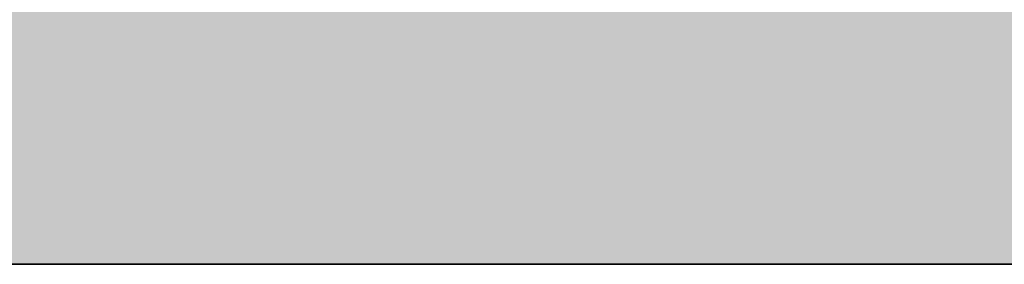
# Model space of a CAD drawing. Units: inches. Extents: x 2083 to 3317, y 1141 to 2115.
# Tile 157 of 256: x 3126.955939 to 3126.958245, y 1263.26136 to 1263.261932. Entities that reach past the tile are written whole.
import ezdxf

# ---------------------------------------------------------------- set-up
doc = ezdxf.new("R2010")
doc.units = ezdxf.units.IN
doc.layers.add('A-ANNO-DIMS', color=2, linetype='Continuous', lineweight=18)
doc.layers.add('A-WALL', color=7, linetype='Continuous', lineweight=35)
doc.layers.add('A-WALL-PATT', color=251, linetype='Continuous', lineweight=13, true_color=0x636466)
doc.styles.get("Standard").update_dxf_attribs({"font": 'arial.ttf'})
doc.dimstyles.new('ISO-25', dxfattribs={"dimtxt": 12, "dimasz": 12, "dimexe": 1.25, "dimexo": 0.625, "dimtad": 1, "dimlunit": 3, "dimtxsty": 'Standard', "dimcen": 2.5, "dimadec": 0, "dimazin": 0, "dimtfac": 1, "dimtmove": 0, "dimatfit": 3, "dimfxl": 1, "dimarcsym": 0})

# ---------------------------------------------------------------- blocks, each defined once
blk = doc.blocks.new('*D10')
at = {"layer": 'A-ANNO-DIMS', "color": 0, "lineweight": -2, "transparency": 16777216}
for p, q in [((2862.9597832, 1262.6363601), (2862.9597832, 1201.3844498)), ((3126.9597832, 1262.6363601), (3126.9597832, 1201.3844498)), ((2874.9597832, 1202.6344498), (3114.9597832, 1202.6344498))]:
    blk.add_line(p, q, dxfattribs=at)
at = {"layer": 'A-ANNO-DIMS', "color": 0, "transparency": 16777216}
for points in [[(2874.9597832, 1204.6344498), (2874.9597832, 1200.6344498), (2862.9597832, 1202.6344498)], [(3114.9597832, 1204.6344498), (3114.9597832, 1200.6344498), (3126.9597832, 1202.6344498)]]:
    blk.add_solid(points, dxfattribs=at)
at = {"layer": 'Defpoints', "color": 0, "transparency": 16777216}
for p in [(2862.9597832, 1263.2613601), (3126.9597832, 1263.2613601), (3126.9597832, 1202.6344498)]:
    blk.add_point(p, dxfattribs=at)
at = {"layer": 'A-ANNO-DIMS', "color": 0, "transparency": 16777216, "insert": (2994.9597832, 1209.2840064), "char_height": 12, "attachment_point": 5}
blk.add_mtext("22'", dxfattribs=at)

msp = doc.modelspace()

# ---------------------------------------------------------------- hatches: boundary and pattern name
at = {"layer": 'A-WALL-PATT'}
h = msp.add_hatch(color=256, dxfattribs=at)
h.dxf.hatch_style = 1
h.paths.add_polyline_path([(3126.9597832, 2020.7613601), (2748.9597832, 2020.7613601), (2604.9597832, 2020.7613601), (2226.9597832, 2020.7613601), (2226.9597832, 1702.7613601), (2466.9597832, 1702.7613601), (2466.9597832, 1582.7613601), (2418.9597832, 1582.7613601), (2418.9597832, 1477.7613601), (2226.9597832, 1477.7613601), (2226.9597832, 1263.2613601), (2544.9597832, 1263.2613601), (2544.9597832, 1411.7613601), (2604.9597832, 1411.7613601), (2685.9597832, 1411.7613601), (2685.9597832, 1420.7613601), (2604.9597832, 1420.7613601), (2604.9597832, 1573.7613601), (2604.9597832, 1702.7613601), (2604.9597832, 2011.7613601), (2748.9597832, 2011.7613601), (2748.9597832, 1702.7613601), (2862.9597832, 1702.7613601), (2862.9597832, 1621.7613601), (2871.9597832, 1621.7613601), (2871.9597832, 1702.7613601), (2883.9597832, 1702.7613601), (2883.9597832, 1706.9394595, -0.026459), (2883.9597832, 1711.7613601), (2757.9597832, 1711.7613601), (2757.9597832, 1807.7613601), (2787.9597832, 1807.7613601), (2787.9597832, 1812.2613601), (2757.9597832, 1812.2613601), (2757.9597832, 2011.7613601), (2877.9597832, 2011.7613601), (2877.9597832, 1812.2613601), (2847.9597832, 1812.2613601), (2847.9597832, 1807.7613601), (2889.8357425, 1807.7613601), (2889.8357425, 1812.2613601), (2882.4597832, 1812.2613601), (2882.4597832, 2011.7613601), (3117.9597832, 2011.7613601), (3117.9597832, 1812.2613601), (2937.8357425, 1812.2613601), (2937.8357425, 1807.7613601), (2995.7097832, 1807.7613601), (2995.7097832, 1796.1176655), (3000.2097832, 1796.1176655), (3000.2097832, 1807.7613601), (3117.9597832, 1807.7613601), (3117.9597832, 1711.7613601), (3000.2097832, 1711.7613601), (3000.2097832, 1760.1176655), (2998.5727047, 1760.1176655, -0.020711), (2995.7097832, 1760.1176655), (2995.7097832, 1711.7613601), (2931.9597832, 1711.7613601), (2931.9597832, 1702.7613601), (3126.9597832, 1702.7613601)])
h.paths.add_polyline_path([(2471.4597832, 2011.7613601), (2471.4597832, 1810.0113601), (2462.7169357, 1810.0113601), (2462.7169357, 1805.5113601), (2505.9597832, 1805.5113601), (2505.9597832, 1810.0113601), (2475.9597832, 1810.0113601), (2475.9597832, 2011.7613601), (2595.9597832, 2011.7613601), (2595.9597832, 1810.0113601), (2565.9597832, 1810.0113601), (2565.9597832, 1805.5113601), (2595.9597832, 1805.5113601), (2595.9597832, 1711.7613601), (2235.9597832, 1711.7613601), (2235.9597832, 1805.5113601), (2353.7097832, 1805.5113601), (2353.7097832, 1796.0541624), (2358.2097832, 1796.0541624), (2358.2097832, 1805.5113601), (2414.7169357, 1805.5113601), (2414.7169357, 1810.0113601), (2235.9597832, 1810.0113601), (2235.9597832, 2011.7613601)], flags=16)
h.paths.add_polyline_path([(2270.2047343, 1994.6100082), (2270.2047343, 1970.6100082), (2246.2047343, 1970.6100082), (2246.2047343, 1994.6100082)], flags=0)
edge = h.paths.add_edge_path(flags=0)
edge.add_ellipse((2332.027391, 1899.7981761), major_axis=(-3.0429938, 3.0429938), ratio=0.16825245, start_angle=-161.3321656, end_angle=-156.3071136, ccw=False)
edge.add_ellipse((2333.0820373, 1898.7435297), major_axis=(-1.0546463, 1.0546463), ratio=0.453532097, start_angle=-123.371019, end_angle=-94.1591066)
edge = h.paths.add_edge_path(flags=0)
edge.add_ellipse((2332.027391, 1968.8762897), major_axis=(3.0429938, 3.0429938), ratio=0.16825245, start_angle=18.6678344, end_angle=23.6928864)
edge.add_spline(control_points=[(2332.9255964, 1970.6911045), (2332.2267681, 1970.3360997), (2330.8937087, 1969.6589054), (2328.4130803, 1970.9321376), (2327.2039345, 1967.7487119), (2324.7095965, 1969.9555886), (2322.5328223, 1967.012354), (2320.0128462, 1971.2958124), (2317.6803077, 1968.1578449), (2316.0405263, 1967.1020468), (2315.4269045, 1966.8096022)], knot_values=[0, 0, 0, 0, 2.267059, 4.324559, 6.685584, 8.878641, 11.121502, 14.300359, 17.755284, 19.732645, 19.732645, 19.732645, 19.732645], degree=3, periodic=0)
edge.add_ellipse((2332.027391, 1968.8762897), major_axis=(3.0429938, 3.0429938), ratio=0.16825245, start_angle=18.6678344, end_angle=23.6928864, ccw=False)
edge.add_ellipse((2333.0820373, 1969.930936), major_axis=(1.0546463, 1.0546463), ratio=0.453532097, start_angle=56.628981, end_angle=85.8408934, ccw=False)
edge = h.paths.add_edge_path(flags=0)
edge.add_spline(control_points=[(2296.4282874, 1967.9879081), (2293.6278045, 1965.3363137), (2287.7036238, 1959.727094), (2299.7438601, 1949.9956993), (2294.5325909, 1935.6685275), (2290.5732281, 1920.6035119), (2293.3941244, 1909.9736911), (2296.1854073, 1904.9665431)], knot_values=[0.099185, 0.099185, 0.099185, 0.099185, 0.345301, 0.619822, 0.982653, 1.386093, 1.810555, 1.810555, 1.810555, 1.810555], degree=3, periodic=0)
edge.add_spline(control_points=[(2296.1854073, 1904.9665431), (2297.3835817, 1902.6193002), (2298.0009694, 1901.9493116), (2298.5529698, 1901.4681549)], knot_values=[0.006246, 0.006246, 0.006246, 0.006246, 0.055476, 0.055476, 0.055476, 0.055476], degree=3, periodic=0)
edge.add_spline(control_points=[(2298.5529698, 1901.4681549), (2297.2586121, 1900.9232238), (2295.2252939, 1900.2321257), (2293.0602287, 1900.6142053), (2292.1014227, 1900.788415), (2292.0895776, 1900.790568)], knot_values=[0.312835, 0.312835, 0.312835, 0.312835, 0.40178, 0.474987, 0.475903, 0.475903, 0.475903, 0.475903], degree=3, periodic=0)
edge.add_arc((2292.7936464, 1904.6641088), 3.9370079, 215.4208969, 259.6981795, ccw=False)
edge.add_spline(control_points=[(2289.5853139, 1902.3823039), (2289.4766524, 1902.5350874), (2289.3684805, 1902.6880353), (2289.2608648, 1902.8411699)], knot_values=[0.102872, 0.102872, 0.102872, 0.102872, 0.116896, 0.116896, 0.116896, 0.116896], degree=3, periodic=0)
edge.add_spline(control_points=[(2289.2608648, 1902.8411699), (2288.6866042, 1902.5501922), (2287.6400477, 1902.0199025), (2285.8813368, 1901.8739536), (2283.8529717, 1901.5043521), (2281.7199871, 1899.7105375), (2278.4669913, 1899.492942), (2276.1571361, 1901.8832022), (2272.2589526, 1899.8040711), (2267.7776054, 1901.8431828), (2262.2438819, 1900.1840326), (2257.414927, 1901.7820606), (2254.318374, 1900.7261196), (2253.1782849, 1900.3373431)], knot_values=[0, 0, 0, 0, 1.907977, 3.477176, 5.261074, 7.972851, 11.680248, 13.717921, 16.939592, 22.789562, 27.502503, 33.595215, 37.145618, 37.145618, 37.145618, 37.145618], degree=3, periodic=0)
edge.add_line((2253.1782849, 1900.3373431), (2250.2442397, 1902.8411699))
edge.add_line((2250.2442397, 1902.8411699), (2250.2442397, 1965.8332959))
edge.add_line((2250.2442397, 1965.8332959), (2253.1782849, 1968.3371226))
edge.add_spline(control_points=[(2253.1782849, 1968.3371226), (2254.318374, 1967.9483462), (2257.414927, 1966.8924051), (2262.2438819, 1968.4904332), (2267.7776054, 1966.8312829), (2271.5267301, 1968.5372172), (2273.8759143, 1967.8282895), (2274.2067012, 1967.7276424)], knot_values=[0, 0, 0, 0, 0.09018, 0.244935, 0.364644, 0.513233, 0.537855, 0.537855, 0.537855, 0.537855], degree=3, periodic=0)
edge.add_arc((2274.3528869, 1963.7933495), 3.9370079, 72.0511336, 92.1279492, ccw=False)
edge.add_arc((2281.2969331, 1985.2300027), 18.5962982, 252.05113361, 288.56572166)
edge.add_arc((2292.3167172, 1956.0288805), 12.6460805, 71.02678788, 113.77821843, ccw=False)
edge = h.paths.add_edge_path(flags=0)
edge.add_spline(control_points=[(2274.8994147, 1951.8561946), (2275.066156, 1951.6165924), (2275.2326866, 1951.3765878), (2275.3979871, 1951.1358545)], knot_values=[1.409916, 1.409916, 1.409916, 1.409916, 1.43159, 1.43159, 1.43159, 1.43159], degree=3, periodic=0)
edge.add_spline(control_points=[(2275.3979871, 1951.1358545), (2275.7921055, 1950.5618854), (2276.1792311, 1949.9837745), (2276.5455462, 1949.3971029)], knot_values=[1.358238, 1.358238, 1.358238, 1.358238, 1.409916, 1.409916, 1.409916, 1.409916], degree=3, periodic=0)
edge.add_line((2276.5455462, 1949.3971029), (2277.437289, 1947.8621847))
edge.add_spline(control_points=[(2277.437289, 1947.8621847), (2276.3038341, 1945.6731147), (2274.6396979, 1942.4268817), (2274.631615, 1938.0938998), (2272.7991237, 1930.8515498), (2274.3564261, 1943.8970461), (2275.9476814, 1947.9233558), (2276.5455462, 1949.3971029)], knot_values=[0.005632, 0.005632, 0.005632, 0.005632, 0.186014, 0.266002, 0.357087, 0.59639, 0.739732, 0.739732, 0.739732, 0.739732], degree=3, periodic=0)
edge.add_spline(control_points=[(2276.5455462, 1949.3971029), (2276.1792311, 1949.9837745), (2275.7921055, 1950.5618854), (2275.3979871, 1951.1358545)], knot_values=[1.358238, 1.358238, 1.358238, 1.358238, 1.409916, 1.409916, 1.409916, 1.409916], degree=3, periodic=0)
edge.add_spline(control_points=[(2275.3979871, 1951.1358545), (2274.9425002, 1950.0804523), (2274.2077604, 1948.0252718), (2273.9346018, 1944.8514774), (2272.4685341, 1937.6274891), (2273.4662155, 1945.6964663), (2274.7006154, 1951.0594725), (2274.8994147, 1951.8561946)], knot_values=[0.104364, 0.104364, 0.104364, 0.104364, 0.189636, 0.269624, 0.36071, 0.600013, 0.644622, 0.644622, 0.644622, 0.644622], degree=3, periodic=0)
h.paths.add_polyline_path([(2269.1675139, 1963.1275729, -0.357527), (2268.170633, 1960.9763695, -0.092561), (2268.170633, 1939.4363249, -0.357527), (2269.1675139, 1937.2851215, -0.357527), (2267.0163105, 1938.2820024, -0.164785), (2254.6855813, 1938.2820024, -0.357527), (2252.5343779, 1937.2851215, -0.357527), (2253.5312587, 1939.4363249, -0.092561), (2253.5312587, 1960.9763695, -0.357527), (2252.5343779, 1963.1275729, -0.357527), (2254.6855813, 1962.130692, -0.164785), (2267.0163105, 1962.130692, -0.357527)], flags=0)
h.paths.add_polyline_path([(2248.8740679, 1967.8017998), (2248.8740679, 1957.0277095), (2249.4577833, 1957.0277095), (2249.4577833, 1911.6467562), (2248.8740679, 1911.6467562), (2248.8740679, 1900.8726659), (2246.5118632, 1900.8726659, 0.197327), (2244.1496584, 1902.4568734), (2244.1496584, 1966.2175923, 0.197327), (2246.5118632, 1967.8017998)], flags=0)
h.paths.add_polyline_path([(2269.1675139, 1931.3893442, -0.357527), (2268.170633, 1929.2381408, -0.092561), (2268.170633, 1907.6980962, -0.357527), (2269.1675139, 1905.5468928, -0.357527), (2267.0163105, 1906.5437737, -0.164785), (2254.6855813, 1906.5437737, -0.357527), (2252.5343779, 1905.5468928, -0.357527), (2253.5312587, 1907.6980962, -0.092561), (2253.5312587, 1929.2381408, -0.357527), (2252.5343779, 1931.3893442, -0.357527), (2254.6855813, 1930.3924634, -0.164785), (2267.0163105, 1930.3924634, -0.357527)], flags=0)
edge = h.paths.add_edge_path(flags=0)
edge.add_spline(control_points=[(2276.1968578, 1906.7237016), (2276.1681442, 1909.0289278), (2276.1140492, 1913.371852), (2270.5984171, 1924.9249783), (2273.9051746, 1919.0127787), (2275.9217115, 1916.2620626), (2275.4745699, 1912.4021495), (2277.2578735, 1910.3806206), (2276.6960436, 1908.2250358), (2276.6462176, 1906.8130226), (2276.6178249, 1906.0084068)], knot_values=[0, 0, 0, 0, 8.61026, 16.221274, 18.843057, 23.804898, 27.440828, 29.356102, 31.203478, 33.650687, 33.650687, 33.650687, 33.650687], degree=3, periodic=0)
edge.add_spline(control_points=[(2276.6178249, 1906.0084068), (2276.6233131, 1905.6241436), (2276.4977381, 1904.6286608), (2275.4417789, 1903.8547251), (2274.9373144, 1903.0804497), (2274.8590804, 1902.8411699)], knot_values=[0.156488, 0.156488, 0.156488, 0.156488, 0.184398, 0.231376, 0.250598, 0.250598, 0.250598, 0.250598], degree=3, periodic=0)
edge.add_line((2274.8590804, 1902.8411699), (2276.50598, 1902.8411699))
edge.add_spline(control_points=[(2276.50598, 1902.8411699), (2276.7883084, 1903.0849395), (2277.6650711, 1904.1251958), (2278.2495378, 1904.340738), (2277.6538719, 1908.5273866), (2278.15567, 1906.2278078), (2278.100464, 1905.2859484), (2278.8466748, 1904.0690054), (2277.8567853, 1903.4149482), (2277.8741909, 1902.9910497), (2277.9035616, 1902.8411699)], knot_values=[0.059574, 0.059574, 0.059574, 0.059574, 0.080753, 0.103741, 0.16972, 0.176036, 0.207137, 0.240474, 0.262341, 0.27366, 0.27366, 0.27366, 0.27366], degree=3, periodic=0)
edge.add_line((2277.9035616, 1902.8411699), (2280.0298255, 1902.8411699))
edge.add_spline(control_points=[(2280.0298255, 1902.8411699), (2279.8882214, 1903.088398), (2279.4992571, 1903.9815512), (2280.1522839, 1905.9393491), (2278.103615, 1909.6577572), (2279.7623946, 1907.185285), (2280.3279002, 1904.8748608), (2280.4851086, 1903.4895904), (2281.4632687, 1903.2494323), (2281.7583431, 1902.9364967), (2281.8340361, 1902.8411699)], knot_values=[0.013856, 0.013856, 0.013856, 0.013856, 0.034874, 0.088867, 0.107879, 0.126738, 0.158714, 0.193757, 0.217487, 0.226722, 0.226722, 0.226722, 0.226722], degree=3, periodic=0)
edge.add_spline(control_points=[(2281.8340361, 1902.8411699), (2281.7875348, 1902.8267029), (2281.6470224, 1902.7829881), (2281.3955272, 1902.85949), (2281.088077, 1902.9852418), (2280.7206826, 1903.060902), (2280.3334513, 1903.0257257), (2280.1247668, 1902.898879), (2280.0298255, 1902.8411699)], knot_values=[0, 0, 0, 0, 0.14413, 0.435517, 0.749276, 1.153046, 1.548371, 1.878348, 1.878348, 1.878348, 1.878348], degree=3, periodic=0)
edge.add_line((2280.0298255, 1902.8411699), (2277.9035616, 1902.8411699))
edge.add_spline(control_points=[(2277.9035616, 1902.8411699), (2277.892855, 1902.7958553), (2277.865396, 1902.6796374), (2277.6074793, 1902.6874828), (2277.2740503, 1902.8006999), (2276.8379209, 1902.6197745), (2276.5838074, 1902.7892611), (2276.50598, 1902.8411699)], knot_values=[0, 0, 0, 0, 0.127189, 0.326199, 0.628009, 1.24357, 1.515331, 1.515331, 1.515331, 1.515331], degree=3, periodic=0)
edge.add_line((2276.50598, 1902.8411699), (2274.8590804, 1902.8411699))
edge.add_spline(control_points=[(2274.8590804, 1902.8411699), (2274.8144367, 1902.8985868), (2274.7251297, 1903.013446), (2274.4934765, 1903.1189684), (2274.2442854, 1902.9605386), (2273.9371207, 1903.1849416), (2273.6140395, 1902.9831428), (2273.4083164, 1902.8830449), (2273.322254, 1902.8411699)], knot_values=[0, 0, 0, 0, 0.21843, 0.436957, 0.687977, 0.990379, 1.398396, 1.69185, 1.69185, 1.69185, 1.69185], degree=3, periodic=0)
edge.add_spline(control_points=[(2273.322254, 1902.8411699), (2273.6167403, 1903.445692), (2274.2739977, 1904.5382529), (2276.0272387, 1904.5737017), (2276.2069634, 1906.5836372), (2276.1968578, 1906.7237016)], knot_values=[0.012227, 0.012227, 0.012227, 0.012227, 0.059472, 0.106218, 0.134458, 0.134458, 0.134458, 0.134458], degree=3, periodic=0)
h.paths.add_polyline_path([(2270.7760538, 1897.7898284), (2270.7760538, 1873.7898284), (2246.7760538, 1873.7898284), (2246.7760538, 1897.7898284)], flags=0)
h.paths.add_polyline_path([(2353.7097832, 1760.0050593), (2353.7097832, 1760.0541624), (2358.2097832, 1760.0541624, -0.033729)], flags=0)
h.paths.add_polyline_path([(2321.8191188, 1737.5291862), (2341.9953271, 1737.5291862, -0.414214), (2343.2032727, 1736.3212406), (2343.2032727, 1721.0205964, -0.414214), (2341.9953271, 1719.8126508), (2321.8191188, 1719.8126508, -0.414214), (2320.6111732, 1721.0205964), (2320.6111732, 1736.3212406, -0.414214)], flags=0)
h.paths.add_polyline_path([(2324.2350099, 1736.3212406), (2339.5794359, 1736.3212406, -0.414214), (2341.9953271, 1733.9053494), (2341.9953271, 1725.4497302, -0.414214), (2339.5794359, 1723.033839), (2333.6805885, 1723.033839), (2333.8453172, 1722.0454666, -0.870646), (2335.4253988, 1721.8258934, -0.767327), (2333.922694, 1721.4232449), (2331.2910241, 1721.4232449, -0.767327), (2329.7883193, 1721.8258934, -0.870646), (2331.3684009, 1722.0454666), (2331.5331296, 1723.033839), (2324.2350099, 1723.033839, -0.414214), (2321.8191188, 1725.4497302), (2321.8191188, 1733.9053494, -0.414214)], flags=0)
h.paths.add_polyline_path([(2570.4837892, 1928.6154443), (2589.6837892, 1928.6154443), (2590.1688286, 1928.6154443), (2590.1688286, 1904.9933971), (2570.4837892, 1904.9933971)], flags=0)
h.paths.add_polyline_path([(2574.4473242, 1927.2638215, -1), (2572.8288357, 1927.2638215, -1)], flags=0)
h.paths.add_polyline_path([(2573.0898665, 1926.9408768), (2573.925032, 1927.7760423), (2574.1477428, 1927.5533315), (2573.3125773, 1926.718166)], flags=0)
h.paths.add_polyline_path([(2578.7790648, 1919.7296175, -1), (2571.5916632, 1919.7296175, -1)], flags=0)
h.paths.add_polyline_path([(2578.385364, 1919.7296175, -1), (2571.985364, 1919.7296175, -1)], flags=0)
h.paths.add_polyline_path([(2331.5957638, 1729.4762156, -1), (2333.6179542, 1729.4762156, -1)], flags=0)
h.paths.add_polyline_path([(2578.0342282, 1927.2638215, -1), (2576.4157396, 1927.2638215, -1)], flags=0)
h.paths.add_polyline_path([(2576.6888513, 1927.5310886), (2576.9115621, 1927.7537993), (2577.7467276, 1926.9186339), (2577.5240168, 1926.6959231)], flags=0)
h.paths.add_polyline_path([(2578.1390648, 1909.8595388, -1), (2572.2316632, 1909.8595388, -1)], flags=0)
h.paths.add_polyline_path([(2577.745364, 1909.8595388, -1), (2572.625364, 1909.8595388, -1)], flags=0)
h.paths.add_polyline_path([(2583.7977179, 1927.2638215, -1), (2582.1792294, 1927.2638215, -1)], flags=0)
h.paths.add_polyline_path([(2582.7186487, 1927.7537993), (2583.5538142, 1926.9186339), (2583.3311034, 1926.6959231), (2582.4959379, 1927.5310886)], flags=0)
h.paths.add_polyline_path([(2582.4959379, 1927.5310886), (2582.7186487, 1927.7537993), (2583.5538142, 1926.9186339), (2583.3311034, 1926.6959231)], flags=0)
h.paths.add_polyline_path([(2587.7390648, 1920.5296175, -1), (2581.8316632, 1920.5296175, -1)], flags=0)
h.paths.add_polyline_path([(2587.345364, 1920.5296175, -1), (2582.225364, 1920.5296175, -1)], flags=0)
h.paths.add_polyline_path([(2587.3846219, 1927.2638215, -1), (2585.7661333, 1927.2638215, -1)], flags=0)
h.paths.add_polyline_path([(2586.0819925, 1926.9802469), (2586.917158, 1927.8154124), (2587.1398688, 1927.5927016), (2586.3047033, 1926.7575361)], flags=0)
h.paths.add_polyline_path([(2588.3790648, 1910.6595388, -1), (2581.1916632, 1910.6595388, -1)], flags=0)
h.paths.add_polyline_path([(2587.985364, 1910.6595388, -1), (2581.585364, 1910.6595388, -1)], flags=0)
h.paths.add_polyline_path([(2417.1677288, 1729.4778955), (2437.3439372, 1729.4778955, -0.414214), (2438.5518828, 1728.2699499), (2438.5518828, 1712.9693057, -0.414214), (2437.3439372, 1711.7613601), (2417.1677288, 1711.7613601, -0.414214), (2415.9597832, 1712.9693057), (2415.9597832, 1728.2699499, -0.414214)], flags=0)
h.paths.add_polyline_path([(2419.58362, 1728.2699499), (2434.928046, 1728.2699499, -0.414214), (2437.3439372, 1725.8540587), (2437.3439372, 1717.3984395, -0.414214), (2434.928046, 1714.9825483), (2429.0291985, 1714.9825483), (2429.1939273, 1713.9941758, -0.870646), (2430.7740089, 1713.7746027, -0.767327), (2429.2713041, 1713.3719542), (2426.6396342, 1713.3719542, -0.767327), (2425.1369294, 1713.7746027, -0.870646), (2426.717011, 1713.9941758), (2426.8817397, 1714.9825483), (2419.58362, 1714.9825483, -0.414214), (2417.1677288, 1717.3984395), (2417.1677288, 1725.8540587, -0.414214)], flags=0)
h.paths.add_polyline_path([(2419.58362, 1728.2699499), (2434.928046, 1728.2699499, -0.414214), (2437.3439372, 1725.8540587), (2437.3439372, 1717.3984395, -0.414214), (2434.928046, 1714.9825483), (2429.0291985, 1714.9825483), (2428.3581177, 1719.0090337), (2427.5528206, 1719.0090337), (2426.8817397, 1714.9825483), (2419.58362, 1714.9825483, -0.414214), (2417.1677288, 1717.3984395), (2417.1677288, 1725.8540587, -0.414214)], flags=0)
h.paths.add_polyline_path([(2426.9443739, 1721.4249248, -1), (2428.9665643, 1721.4249248, -1)], flags=0)
h.paths.add_polyline_path([(2475.9597832, 1702.7613601), (2595.9597832, 1702.7613601), (2595.9597832, 1582.7613601), (2475.9597832, 1582.7613601)], flags=16)
h.paths.add_polyline_path([(2427.9597832, 1573.7613601), (2595.9597832, 1573.7613601), (2595.9597832, 1468.7613601), (2595.9597832, 1420.7613601), (2384.4597832, 1420.7613601), (2384.4597832, 1468.7613601), (2427.9597832, 1468.7613601)], flags=16)
h.paths.add_polyline_path([(2379.9597832, 1468.7613601), (2379.9597832, 1420.7613601), (2235.9597832, 1420.7613601), (2235.9597832, 1468.7613601)], flags=16)
h.paths.add_polyline_path([(2317.8159962, 1466.695767), (2337.9922045, 1466.695767, -0.414214), (2339.2001501, 1465.4878214), (2339.2001501, 1450.1871771, -0.414214), (2337.9922045, 1448.9792315), (2317.8159962, 1448.9792315, -0.414214), (2316.6080506, 1450.1871771), (2316.6080506, 1465.4878214, -0.414214)], flags=0)
h.paths.add_polyline_path([(2320.2318874, 1465.4878214), (2335.5763133, 1465.4878214, -0.414214), (2337.9922045, 1463.0719302), (2337.9922045, 1454.616311, -0.414214), (2335.5763133, 1452.2004198), (2329.6774659, 1452.2004198), (2329.8421946, 1451.2120473, -0.870646), (2331.4222762, 1450.9924742, -0.767327), (2329.9195714, 1450.5898257), (2327.2879015, 1450.5898257, -0.767327), (2325.7851967, 1450.9924742, -0.870646), (2327.3652783, 1451.2120473), (2327.530007, 1452.2004198), (2320.2318874, 1452.2004198, -0.414214), (2317.8159962, 1454.616311), (2317.8159962, 1463.0719302, -0.414214)], flags=0)
h.paths.add_polyline_path([(2320.2318874, 1465.4878214), (2335.5763133, 1465.4878214, -0.414214), (2337.9922045, 1463.0719302), (2337.9922045, 1454.616311, -0.414214), (2335.5763133, 1452.2004198), (2329.6774659, 1452.2004198), (2329.006385, 1456.2269051), (2328.2010879, 1456.2269051), (2327.530007, 1452.2004198), (2320.2318874, 1452.2004198, -0.414214), (2317.8159962, 1454.616311), (2317.8159962, 1463.0719302, -0.414214)], flags=0)
h.paths.add_polyline_path([(2327.5926413, 1458.6427963, -1), (2329.6148317, 1458.6427963, -1)], flags=0)
h.paths.add_polyline_path([(2244.4117436, 1433.3404531), (2241.9209449, 1433.3404531, -0.414214), (2240.0178562, 1435.2435418), (2240.0178562, 1440.9528078, -0.414211), (2241.920925, 1442.8558965), (2244.4117436, 1442.8558965, -1.976472)], flags=0)
h.paths.add_polyline_path([(2245.3568884, 1434.3975358, -0.414214), (2245.3568884, 1441.7988138, -2.144098)], flags=0)
h.paths.add_polyline_path([(2535.9597832, 1416.2613601), (2535.9597832, 1272.2613601), (2235.9597832, 1272.2613601), (2235.9597832, 1416.2613601)], flags=16)
h.paths.add_polyline_path([(2260.1195614, 1384.2928413), (2260.1195614, 1362.0386487), (2237.8653688, 1362.0386487), (2237.8653688, 1384.2928413)], flags=0)
edge = h.paths.add_edge_path(flags=0)
edge.add_line((2318.2518466, 1362.0932983), (2318.1457968, 1362.0009726))
edge.add_ellipse((2317.4451158, 1360.4310442), major_axis=(2.8216404, 2.8216404), ratio=0.16825245, start_angle=18.6678344, end_angle=20.9481273, ccw=False)
edge.add_ellipse((2318.4230451, 1361.4089735), major_axis=(0.9779293, 0.9779293), ratio=0.453532097, start_angle=56.628981, end_angle=70.2262012, ccw=False)
edge = h.paths.add_edge_path(flags=0)
edge.add_line((2319.1073699, 1295.5710784), (2319.0150442, 1295.6771282))
edge.add_ellipse((2317.4451158, 1296.3778091), major_axis=(-2.8216404, 2.8216404), ratio=0.16825245, start_angle=-161.3321656, end_angle=-159.0518727, ccw=False)
edge.add_ellipse((2318.4230451, 1295.3998798), major_axis=(-0.9779293, 0.9779293), ratio=0.453532097, start_angle=-123.371019, end_angle=-109.7737988)
edge = h.paths.add_edge_path(flags=0)
edge.add_spline(control_points=[(2284.2103489, 1301.1702189), (2284.5806878, 1300.444719), (2284.8911891, 1299.8920243), (2285.159553, 1299.4610182)], knot_values=[0.039066, 0.039066, 0.039066, 0.039066, 0.055476, 0.055476, 0.055476, 0.055476], degree=3, periodic=0)
edge.add_line((2285.159553, 1299.4610182), (2284.2103489, 1301.1702189))
edge = h.paths.add_edge_path(flags=0)
edge.add_line((2280.4124579, 1297.2980125), (2283.3699905, 1297.0361216))
edge.add_line((2283.3699905, 1297.0361216), (2286.4056902, 1297.9263104))
edge.add_spline(control_points=[(2286.4056902, 1297.9263104), (2285.305487, 1297.4631193), (2284.3447774, 1297.1291508), (2283.3699905, 1297.0361216)], knot_values=[0.394369, 0.394369, 0.394369, 0.394369, 0.475903, 0.475903, 0.475903, 0.475903], degree=3, periodic=0)
edge.add_spline(control_points=[(2283.3699905, 1297.0361216), (2283.2813895, 1297.027666), (2282.316289, 1296.9573356), (2281.3125019, 1297.1344787), (2280.4234414, 1297.2960161), (2280.4124579, 1297.2980125)], knot_values=[0.312835, 0.312835, 0.312835, 0.312835, 0.320246, 0.393453, 0.394369, 0.394369, 0.394369, 0.394369], degree=3, periodic=0)
edge = h.paths.add_edge_path(flags=0)
edge.add_line((2284.4355615, 1359.6072854), (2280.4462909, 1355.328047))
edge.add_line((2280.4462909, 1355.328047), (2279.5799868, 1351.0177544))
edge.add_line((2279.5799868, 1351.0177544), (2282.4129737, 1346.5804327))
edge.add_spline(control_points=[(2282.4129737, 1346.5804327), (2283.1533308, 1345.5892358), (2284.2528957, 1344.0288973), (2284.801037, 1342.3871671), (2284.9351625, 1341.8055443)], knot_values=[1.240098, 1.240098, 1.240098, 1.240098, 1.332892, 1.382712, 1.382712, 1.382712, 1.382712], degree=3, periodic=0)
edge.add_spline(control_points=[(2284.9351625, 1341.8055443), (2285.3191079, 1340.1406002), (2285.2330291, 1338.4092041), (2284.9099384, 1336.6541222)], knot_values=[1.097484, 1.097484, 1.097484, 1.097484, 1.240098, 1.240098, 1.240098, 1.240098], degree=3, periodic=0)
edge.add_spline(control_points=[(2284.9099384, 1336.6541222), (2284.5868478, 1334.8990403), (2284.0267453, 1333.1202725), (2283.4626437, 1331.3605849)], knot_values=[0.95487, 0.95487, 0.95487, 0.95487, 1.097484, 1.097484, 1.097484, 1.097484], degree=3, periodic=0)
edge.add_line((2283.4626437, 1331.3605849), (2281.8903759, 1326.153357))
edge.add_line((2281.8903759, 1326.153357), (2280.7562592, 1321.0560888))
edge.add_line((2280.7562592, 1321.0560888), (2280.2992048, 1316.0019772))
edge.add_line((2280.2992048, 1316.0019772), (2280.7159327, 1310.9500678))
edge.add_line((2280.7159327, 1310.9500678), (2282.0280939, 1305.9721367))
edge.add_line((2282.0280939, 1305.9721367), (2284.2103489, 1301.1702189))
edge.add_spline(control_points=[(2284.2103489, 1301.1702189), (2283.3407305, 1302.7301854), (2282.6119044, 1304.3364933), (2282.0280939, 1305.9721367)], knot_values=[0.099185, 0.099185, 0.099185, 0.099185, 0.241799, 0.241799, 0.241799, 0.241799], degree=3, periodic=0)
edge.add_spline(control_points=[(2282.0280939, 1305.9721367), (2281.4442835, 1307.6077801), (2281.0054886, 1309.2727591), (2280.7159327, 1310.9500678)], knot_values=[0.241799, 0.241799, 0.241799, 0.241799, 0.384413, 0.384413, 0.384413, 0.384413], degree=3, periodic=0)
edge.add_spline(control_points=[(2280.7159327, 1310.9500678), (2280.4332411, 1312.5876134), (2280.2893863, 1314.2769594), (2280.2988938, 1315.9620324), (2280.2992048, 1316.0019772)], knot_values=[0.384413, 0.384413, 0.384413, 0.384413, 0.523647, 0.527028, 0.527028, 0.527028, 0.527028], degree=3, periodic=0)
edge.add_spline(control_points=[(2280.2992048, 1316.0019772), (2280.3123257, 1317.6869552), (2280.4778706, 1319.3679256), (2280.7562592, 1321.0560888)], knot_values=[0.527028, 0.527028, 0.527028, 0.527028, 0.669642, 0.669642, 0.669642, 0.669642], degree=3, periodic=0)
edge.add_spline(control_points=[(2280.7562592, 1321.0560888), (2281.0346478, 1322.7442519), (2281.4258801, 1324.4396079), (2281.8903759, 1326.153357)], knot_values=[0.669642, 0.669642, 0.669642, 0.669642, 0.812256, 0.812256, 0.812256, 0.812256], degree=3, periodic=0)
edge.add_spline(control_points=[(2281.8903759, 1326.153357), (2282.2643834, 1327.5332507), (2282.7878702, 1329.2618097), (2283.352751, 1331.0177803), (2283.4626437, 1331.3605849)], knot_values=[0.812256, 0.812256, 0.812256, 0.812256, 0.927087, 0.95487, 0.95487, 0.95487, 0.95487], degree=3, periodic=0)
edge.add_line((2283.4626437, 1331.3605849), (2284.9099384, 1336.6541222))
edge.add_line((2284.9099384, 1336.6541222), (2284.9351625, 1341.8055443))
edge.add_line((2284.9351625, 1341.8055443), (2282.4129737, 1346.5804327))
edge.add_spline(control_points=[(2282.4129737, 1346.5804327), (2281.2751273, 1348.1037918), (2280.0784467, 1349.5703178), (2279.5799868, 1351.0177544)], knot_values=[1.382712, 1.382712, 1.382712, 1.382712, 1.525326, 1.525326, 1.525326, 1.525326], degree=3, periodic=0)
edge.add_spline(control_points=[(2279.5799868, 1351.0177544), (2279.4432818, 1351.4147209), (2279.1363124, 1352.856922), (2279.7351897, 1354.2903851), (2280.4462909, 1355.328047)], knot_values=[1.525326, 1.525326, 1.525326, 1.525326, 1.564439, 1.667941, 1.667941, 1.667941, 1.667941], degree=3, periodic=0)
edge.add_spline(control_points=[(2280.4462909, 1355.328047), (2281.4261132, 1356.7578354), (2282.9308373, 1358.1825604), (2284.4355615, 1359.6072854)], knot_values=[1.667941, 1.667941, 1.667941, 1.667941, 1.810555, 1.810555, 1.810555, 1.810555], degree=3, periodic=0)
edge.add_arc((2280.6230749, 1348.518181), 11.7261796, 71.02678788, 113.77821843)
edge.add_arc((2270.4048917, 1375.5951559), 17.2435667, 252.05113361, 288.56572166, ccw=False)
edge.add_arc((2263.9659692, 1355.7178471), 3.6506221, 72.0511336, 92.1279492)
edge.add_arc((2263.9659692, 1355.7178471), 3.6506221, 92.1279492, 177.98513)
edge.add_spline(control_points=[(2260.3176041, 1355.8461989), (2260.2604169, 1354.2206683), (2260.551278, 1350.1865469), (2262.9993445, 1346.7662507), (2264.4727415, 1344.6490245)], knot_values=[1.43159, 1.43159, 1.43159, 1.43159, 1.564144, 1.770695, 1.770695, 1.770695, 1.770695], degree=3, periodic=0)
edge.add_line((2264.4727415, 1344.6490245), (2264.9355904, 1343.9825301))
edge.add_spline(control_points=[(2263.8010444, 1340.2481052), (2263.8432379, 1340.5140884), (2264.0672444, 1341.7564652), (2264.5126928, 1343.0024532), (2264.9350468, 1343.9810834)], knot_values=[0.53657, 0.53657, 0.53657, 0.53657, 0.559349, 0.644622, 0.644622, 0.644622, 0.644622], degree=3, periodic=0)
edge.add_spline(control_points=[(2264.9350468, 1343.9810834), (2265.1177715, 1343.7149747), (2265.2988751, 1343.4479058), (2265.4767562, 1343.1793646)], knot_values=[1.384077, 1.384077, 1.384077, 1.384077, 1.409916, 1.409916, 1.409916, 1.409916], degree=3, periodic=0)
edge.add_spline(control_points=[(2265.4767562, 1343.1793646), (2265.6546373, 1342.9108234), (2265.8292958, 1342.64081), (2265.9991301, 1342.368812)], knot_values=[1.358238, 1.358238, 1.358238, 1.358238, 1.384077, 1.384077, 1.384077, 1.384077], degree=3, periodic=0)
edge.add_line((2265.9991301, 1342.368812), (2266.8260057, 1340.9455468))
edge.add_spline(control_points=[(2266.8260057, 1340.9455468), (2268.894401, 1337.0896912), (2271.3981727, 1325.8430009), (2270.5161644, 1310.5685568), (2275.9193759, 1301.860609), (2277.7895113, 1299.1994495)], knot_values=[0.116896, 0.116896, 0.116896, 0.116896, 0.472987, 1.050969, 1.313793, 1.313793, 1.313793, 1.313793], degree=3, periodic=0)
edge.add_spline(control_points=[(2277.7895113, 1299.1994495), (2277.8394051, 1299.1284519), (2277.8894277, 1299.0574975), (2277.9395717, 1298.9865839)], knot_values=[0.109884, 0.109884, 0.109884, 0.109884, 0.116896, 0.116896, 0.116896, 0.116896], degree=3, periodic=0)
edge.add_line((2277.9395717, 1298.9865839), (2277.7888489, 1299.1991139))
edge.add_spline(control_points=[(2277.7888489, 1299.1991139), (2277.2565819, 1298.9294144), (2276.2863504, 1298.4379024), (2275.0393517, 1298.3344186), (2274.3833299, 1298.2388951), (2274.2152543, 1298.209338)], knot_values=[33.12187, 33.12187, 33.12187, 33.12187, 35.029056, 36.598255, 37.144827, 37.144827, 37.144827, 37.144827], degree=3, periodic=0)
edge.add_line((2274.2152543, 1298.209338), (2273.073147, 1297.8929607))
edge.add_spline(control_points=[(2273.073147, 1297.8929607), (2272.3229363, 1297.579784), (2271.0391507, 1296.5105078), (2269.2483948, 1296.2260622), (2268.4231004, 1296.3746543)], knot_values=[26.532584, 26.532584, 26.532584, 26.532584, 29.198919, 31.839101, 31.839101, 31.839101, 31.839101], degree=3, periodic=0)
edge.add_line((2268.4231004, 1296.3746543), (2263.8785014, 1297.4575338))
edge.add_spline(control_points=[(2263.8785014, 1297.4575338), (2263.5560769, 1297.3594345), (2261.8603064, 1296.8386943), (2260.2387805, 1297.2824073), (2258.9334543, 1297.5164611)], knot_values=[15.919551, 15.919551, 15.919551, 15.919551, 16.939592, 21.226067, 21.226067, 21.226067, 21.226067], degree=3, periodic=0)
edge.add_line((2258.9334543, 1297.5164611), (2254.0552332, 1297.3290098))
edge.add_spline(control_points=[(2254.0552332, 1297.3290098), (2253.7555255, 1297.295815), (2252.1136834, 1297.1651738), (2250.4618687, 1297.5442209), (2249.1296862, 1297.6678818)], knot_values=[5.306517, 5.306517, 5.306517, 5.306517, 6.276435, 10.613034, 10.613034, 10.613034, 10.613034], degree=3, periodic=0)
edge.add_line((2249.1296862, 1297.6678818), (2244.3316495, 1296.8777561))
edge.add_line((2244.3316495, 1296.8777561), (2241.6110326, 1299.1994495))
edge.add_line((2241.6110326, 1299.1994495), (2241.6110326, 1357.6094038))
edge.add_line((2241.6110326, 1357.6094038), (2244.3316495, 1359.9310973))
edge.add_line((2244.3316495, 1359.9310973), (2252.7288228, 1359.5426917))
edge.add_spline(control_points=[(2252.7288228, 1359.5426917), (2252.8709387, 1359.5464396), (2253.3057402, 1359.5481716), (2253.7398447, 1359.5142744), (2254.0317419, 1359.4824261)], knot_values=[0.233291, 0.233291, 0.233291, 0.233291, 0.244935, 0.268927, 0.268927, 0.268927, 0.268927], degree=3, periodic=0)
edge.add_line((2254.0317419, 1359.4824261), (2259.5871899, 1359.4163899))
edge.add_spline(control_points=[(2259.5871899, 1359.4163899), (2260.6770676, 1359.6285026), (2262.0731971, 1359.8970025), (2263.5236925, 1359.4592776), (2263.8304173, 1359.3659518)], knot_values=[0.422516, 0.422516, 0.422516, 0.422516, 0.513233, 0.537855, 0.537855, 0.537855, 0.537855], degree=3, periodic=0)
edge.add_arc((2263.9659692, 1355.7178471), 3.6506221, 72.0511336, 92.1279492, ccw=False)
edge.add_arc((2270.4048917, 1375.5951559), 17.2435667, 252.05113361, 288.56572166)
edge.add_arc((2280.6230749, 1348.518181), 11.7261796, 71.02678788, 113.77821843, ccw=False)
h.paths.add_polyline_path([(2240.3405298, 1359.4347149), (2240.3405298, 1349.4443532), (2240.8817846, 1349.4443532), (2240.8817846, 1307.3645001), (2240.3405298, 1307.3645001), (2240.3405298, 1297.3741385), (2238.1501565, 1297.3741385, 0.197327), (2235.9597832, 1298.8431076), (2235.9597832, 1357.9657458, 0.197327), (2238.1501565, 1359.4347149)], flags=0)
h.paths.add_polyline_path([(2259.1577904, 1355.1005005, -0.357527), (2258.2334246, 1353.1057799, -0.092561), (2258.2334246, 1333.1326007, -0.357527), (2259.1577904, 1331.1378801, -0.357527), (2257.1630698, 1332.0622458, -0.164785), (2245.7293022, 1332.0622458, -0.357527), (2243.7345816, 1331.1378801, -0.357527), (2244.6589474, 1333.1326007, -0.092561), (2244.6589474, 1353.1057799, -0.357527), (2243.7345816, 1355.1005005, -0.357527), (2245.7293022, 1354.1761347, -0.164785), (2257.1630698, 1354.1761347, -0.357527)], flags=0)
edge = h.paths.add_edge_path(flags=0)
edge.add_line((2265.9991301, 1342.368812), (2266.8260057, 1340.9455468))
edge.add_line((2266.8260057, 1340.9455468), (2265.3075567, 1337.8140664))
edge.add_line((2265.3075567, 1337.8140664), (2264.358232, 1334.6529388))
edge.add_line((2264.358232, 1334.6529388), (2264.2620123, 1333.7997046))
edge.add_spline(control_points=[(2264.2620123, 1333.7997046), (2264.2083565, 1333.187055), (2264.1620602, 1332.3655252), (2264.0071444, 1331.4139326), (2263.9690487, 1331.2018338)], knot_values=[0.464444, 0.464444, 0.464444, 0.464444, 0.516691, 0.531608, 0.531608, 0.531608, 0.531608], degree=3, periodic=0)
edge.add_spline(control_points=[(2263.9690487, 1331.2018338), (2263.7745349, 1330.1188727), (2263.4243703, 1328.7908386), (2263.2574202, 1328.5306516), (2263.2340282, 1328.5146115)], knot_values=[0.372682, 0.372682, 0.372682, 0.372682, 0.44885, 0.464444, 0.464444, 0.464444, 0.464444], degree=3, periodic=0)
edge.add_spline(control_points=[(2263.2340282, 1328.5146115), (2263.096382, 1328.4202271), (2263.1311696, 1329.3014765), (2263.2749528, 1330.6157493)], knot_values=[0.280919, 0.280919, 0.280919, 0.280919, 0.372682, 0.372682, 0.372682, 0.372682], degree=3, periodic=0)
edge.add_spline(control_points=[(2263.2749528, 1330.6157493), (2263.4187361, 1331.930022), (2263.6715151, 1333.677318), (2263.9698519, 1335.3150268)], knot_values=[0.189157, 0.189157, 0.189157, 0.189157, 0.280919, 0.280919, 0.280919, 0.280919], degree=3, periodic=0)
edge.add_spline(control_points=[(2263.9698519, 1335.3150268), (2264.1004958, 1336.0321917), (2264.4187827, 1337.6219113), (2264.7548476, 1338.8644304), (2264.9474193, 1339.4911244)], knot_values=[0.097394, 0.097394, 0.097394, 0.097394, 0.137578, 0.189157, 0.189157, 0.189157, 0.189157], degree=3, periodic=0)
edge.add_spline(control_points=[(2264.9474193, 1339.4911244), (2265.2900171, 1340.6060546), (2265.6442376, 1341.4939958), (2265.9991301, 1342.368812)], knot_values=[0.005632, 0.005632, 0.005632, 0.005632, 0.097394, 0.097394, 0.097394, 0.097394], degree=3, periodic=0)
h.paths.add_polyline_path([(2259.1577904, 1325.6709733, -0.357527), (2258.2334246, 1323.6762527, -0.092561), (2258.2334246, 1303.7030735, -0.357527), (2259.1577904, 1301.7083529, -0.357527), (2257.1630698, 1302.6327186, -0.164785), (2245.7293022, 1302.6327186, -0.357527), (2243.7345816, 1301.7083529, -0.357527), (2244.6589474, 1303.7030735, -0.092561), (2244.6589474, 1323.6762527, -0.357527), (2243.7345816, 1325.6709733, -0.357527), (2245.7293022, 1324.7466075, -0.164785), (2257.1630698, 1324.7466075, -0.357527)], flags=0)
edge = h.paths.add_edge_path(flags=0)
edge.add_spline(control_points=[(2261.7089377, 1317.3114208), (2261.6794818, 1317.4175798), (2261.7618581, 1317.3885347), (2262.4907358, 1316.0898725), (2262.962185, 1315.3008975)], knot_values=[14.955861, 14.955861, 14.955861, 14.955861, 16.221274, 18.694826, 18.694826, 18.694826, 18.694826], degree=3, periodic=0)
edge.add_spline(control_points=[(2262.962185, 1315.3008975), (2262.9904374, 1315.2536169), (2263.7020958, 1314.0673762), (2264.3489834, 1313.1271533), (2264.7300545, 1312.1641544)], knot_values=[18.694826, 18.694826, 18.694826, 18.694826, 18.843057, 22.433791, 22.433791, 22.433791, 22.433791], degree=3, periodic=0)
edge.add_spline(control_points=[(2264.7300545, 1312.1641544), (2264.8755649, 1311.7964373), (2265.1768733, 1310.7698073), (2265.1430689, 1309.5592623), (2265.2477363, 1308.8241926)], knot_values=[22.433791, 22.433791, 22.433791, 22.433791, 23.804898, 26.172756, 26.172756, 26.172756, 26.172756], degree=3, periodic=0)
edge.add_line((2265.2477363, 1308.8241926), (2265.8507741, 1307.1718879))
edge.add_spline(control_points=[(2265.8507741, 1307.1718879), (2266.0650246, 1306.8216779), (2266.3843872, 1306.3322461), (2266.4244001, 1305.7805489), (2266.4203688, 1305.6112163)], knot_values=[28.062562, 28.062562, 28.062562, 28.062562, 29.356102, 29.911721, 29.911721, 29.911721, 29.911721], degree=3, periodic=0)
edge.add_spline(control_points=[(2266.4203688, 1305.6112163), (2266.4161162, 1305.4325896), (2266.393999, 1305.2499979), (2266.3647773, 1305.0658571)], knot_values=[29.911721, 29.911721, 29.911721, 29.911721, 30.497837, 30.497837, 30.497837, 30.497837], degree=3, periodic=0)
edge.add_line((2266.3647773, 1305.0658571), (2266.0661511, 1302.1362954))
edge.add_spline(control_points=[(2266.0661511, 1302.1362954), (2266.0712401, 1301.7799843), (2265.9980761, 1301.1999847), (2265.6632664, 1300.7589613), (2265.5089084, 1300.5858824)], knot_values=[0.156488, 0.156488, 0.156488, 0.156488, 0.184398, 0.203543, 0.203543, 0.203543, 0.203543], degree=3, periodic=0)
edge.add_line((2265.5089084, 1300.5858824), (2264.4353411, 1299.1994495))
edge.add_line((2264.4353411, 1299.1994495), (2265.962442, 1299.1994495))
edge.add_line((2265.962442, 1299.1994495), (2267.3359898, 1301.1752758))
edge.add_line((2267.3359898, 1301.1752758), (2267.3116668, 1301.9862366))
edge.add_spline(control_points=[(2267.3116668, 1301.9862366), (2267.261111, 1302.8623959), (2267.1602121, 1303.7371316), (2267.2714865, 1303.3258962)], knot_values=[0.126229, 0.126229, 0.126229, 0.126229, 0.166617, 0.166617, 0.166617, 0.166617], degree=3, periodic=0)
edge.add_spline(control_points=[(2267.2714865, 1303.3258962), (2267.2800347, 1303.2943047), (2267.3097851, 1303.1753659), (2267.3734504, 1302.8836084), (2267.4061233, 1302.6828291), (2267.4179259, 1302.6010251)], knot_values=[0.166617, 0.166617, 0.166617, 0.166617, 0.16972, 0.176036, 0.180765, 0.180765, 0.180765, 0.180765], degree=3, periodic=0)
edge.add_spline(control_points=[(2267.7438914, 1300.9875045), (2267.6875832, 1301.1509426), (2267.4805198, 1301.6566644), (2267.4837514, 1302.1447877), (2267.4179259, 1302.6010251)], knot_values=[0.180765, 0.180765, 0.180765, 0.180765, 0.193767, 0.220139, 0.220139, 0.220139, 0.220139], degree=3, periodic=0)
edge.add_line((2267.4179259, 1302.6010251), (2267.7438914, 1300.9875045))
edge.add_spline(control_points=[(2267.7438914, 1300.9875045), (2267.8319608, 1300.7318778), (2267.9320205, 1300.3099042), (2267.5548409, 1299.9745185), (2267.429366, 1299.8292073)], knot_values=[0.220139, 0.220139, 0.220139, 0.220139, 0.240474, 0.25489, 0.25489, 0.25489, 0.25489], degree=3, periodic=0)
edge.add_line((2267.429366, 1299.8292073), (2267.2583608, 1299.1994495))
edge.add_line((2267.2583608, 1299.1994495), (2269.229956, 1299.1994495))
edge.add_spline(control_points=[(2269.229956, 1299.1994495), (2269.0986525, 1299.4286938), (2268.842774, 1300.0162509), (2269.0115749, 1300.9159235), (2268.9467957, 1301.6607397)], knot_values=[0.013856, 0.013856, 0.013856, 0.013856, 0.034874, 0.067073, 0.067073, 0.067073, 0.067073], degree=3, periodic=0)
edge.add_line((2268.9467957, 1301.6607397), (2268.4315815, 1303.6031089))
edge.add_spline(control_points=[(2268.4315815, 1303.6031089), (2268.1755957, 1304.1923747), (2267.5962136, 1305.2512977), (2268.0406981, 1304.6232098), (2268.2513938, 1304.2824205)], knot_values=[0.090155, 0.090155, 0.090155, 0.090155, 0.107879, 0.120289, 0.120289, 0.120289, 0.120289], degree=3, periodic=0)
edge.add_spline(control_points=[(2268.2513938, 1304.2824205), (2268.3608818, 1304.1053294), (2269.0577527, 1302.9179833), (2269.382691, 1301.5904186), (2269.5214051, 1300.7759312), (2269.5752202, 1300.5557836)], knot_values=[0.120289, 0.120289, 0.120289, 0.120289, 0.126738, 0.158714, 0.173506, 0.173506, 0.173506, 0.173506], degree=3, periodic=0)
edge.add_line((2269.5752202, 1300.5557836), (2270.6857984, 1299.4212579))
edge.add_spline(control_points=[(2270.6857984, 1299.4212579), (2270.7672206, 1299.3572512), (2270.8378523, 1299.2814011), (2270.9029248, 1299.1994495)], knot_values=[0.21816, 0.21816, 0.21816, 0.21816, 0.226722, 0.226722, 0.226722, 0.226722], degree=3, periodic=0)
edge.add_line((2270.9372012, 1299.1929131), (2270.9029248, 1299.1994495))
edge.add_spline(control_points=[(2270.9029248, 1299.1994495), (2270.8598061, 1299.1860349), (2270.7295148, 1299.1455), (2270.4963139, 1299.216437), (2270.2716612, 1299.3083234), (2270.1210168, 1299.3479612), (2270.0633386, 1299.3595566)], knot_values=[0.939174, 0.939174, 0.939174, 0.939174, 1.083304, 1.374691, 1.68845, 1.878348, 1.878348, 1.878348, 1.878348], degree=3, periodic=0)
edge.add_line((2270.0633386, 1299.3595566), (2269.229956, 1299.1994495))
edge.add_line((2269.229956, 1299.1994495), (2267.2583608, 1299.1994495))
edge.add_spline(control_points=[(2267.2583608, 1299.1994495), (2267.248433, 1299.1574312), (2267.2229714, 1299.0496673), (2266.9838161, 1299.056942), (2266.8092097, 1299.1162303), (2266.6769047, 1299.1090913), (2266.636531, 1299.1048147)], knot_values=[0.757665, 0.757665, 0.757665, 0.757665, 0.884854, 1.083864, 1.385675, 1.515331, 1.515331, 1.515331, 1.515331], degree=3, periodic=0)
edge.add_spline(control_points=[(2266.636531, 1299.1048147), (2266.4852248, 1299.0887878), (2266.2358066, 1299.0171229), (2266.0346081, 1299.1513168), (2265.962442, 1299.1994495)], knot_values=[0, 0, 0, 0, 0.485905, 0.757665, 0.757665, 0.757665, 0.757665], degree=3, periodic=0)
edge.add_line((2265.962442, 1299.1994495), (2264.4353411, 1299.1994495))
edge.add_line((2264.4353411, 1299.1994495), (2263.8584442, 1299.3671176))
edge.add_spline(control_points=[(2263.8584442, 1299.3671176), (2263.8189433, 1299.3709053), (2263.7795277, 1299.3857212), (2263.7401308, 1299.4015039)], knot_values=[0.845925, 0.845925, 0.845925, 0.845925, 0.978627, 0.978627, 0.978627, 0.978627], degree=3, periodic=0)
edge.add_line((2263.7217862, 1299.3964251), (2263.0103065, 1299.1994495))
edge.add_spline(control_points=[(2263.0103065, 1299.1994495), (2263.2457942, 1299.682859), (2263.5060317, 1300.1281072), (2263.8734943, 1300.4080279)], knot_values=[0.012227, 0.012227, 0.012227, 0.012227, 0.052971, 0.052971, 0.052971, 0.052971], degree=3, periodic=0)
edge.add_spline(control_points=[(2263.8734943, 1300.4080279), (2263.932131, 1300.4526954), (2264.0842429, 1300.5529789), (2264.2551889, 1300.6242227), (2264.3596855, 1300.6647475)], knot_values=[0.052971, 0.052971, 0.052971, 0.052971, 0.059472, 0.069086, 0.069086, 0.069086, 0.069086], degree=3, periodic=0)
edge.add_line((2264.3596855, 1300.6647475), (2265.1418998, 1301.0777737))
edge.add_line((2265.1418998, 1301.0777737), (2265.675806, 1302.7995583))
edge.add_line((2265.675806, 1302.7995583), (2265.5407004, 1305.7040662))
edge.add_line((2265.5407004, 1305.7040662), (2264.8030733, 1309.3277237))
edge.add_line((2264.8030733, 1309.3277237), (2263.0405349, 1314.0917906))
edge.add_spline(control_points=[(2263.0405349, 1314.0917906), (2262.3835724, 1315.6714379), (2261.7959724, 1316.9977489), (2261.7089377, 1317.3114208)], knot_values=[11.216896, 11.216896, 11.216896, 11.216896, 14.955861, 14.955861, 14.955861, 14.955861], degree=3, periodic=0)
h.paths.add_polyline_path([(2871.9597832, 1416.2613601), (2895.910047, 1416.2613601), (2895.910047, 1420.7613601), (2871.9597832, 1420.7613601), (2871.9597832, 1501.7613601), (2862.9597832, 1501.7613601), (2862.9597832, 1420.7613601), (2805.9597832, 1420.7613601), (2805.9597832, 1411.7613601), (2862.9597832, 1411.7613601), (2862.9597832, 1263.2613601), (3126.9597832, 1263.2613601), (3126.9597832, 1411.7613601), (3126.9597832, 1486.7613601), (2943.9597832, 1486.7613601), (2943.9597832, 1477.7613601), (2967.8603109, 1477.7613601), (2967.8603109, 1420.7613601), (2943.910047, 1420.7613601), (2943.910047, 1416.2613601), (3117.9597832, 1416.2613601), (3117.9597832, 1420.7613601), (2972.3603109, 1420.7613601), (2972.3603109, 1477.7613601), (3117.9597832, 1477.7613601), (3117.9597832, 1420.7613601), (3117.9597832, 1272.2613601), (2871.9597832, 1272.2613601)], flags=0)
h.paths.add_polyline_path([(2457.1256256, 1485.9425054), (2527.6026508, 1485.9425054), (2527.6026508, 1537.6357021), (2457.1256256, 1537.6357021)], flags=8)
h.paths.add_polyline_path([(2481.0050583, 1609.9818039), (2590.765818, 1609.9818039), (2590.765818, 1682.0033623), (2481.0050583, 1682.0033623)], flags=8)
h.paths.add_polyline_path([(2483.0850224, 1729.1267835), (2553.5620476, 1729.1267835), (2553.5620476, 1780.8199802), (2483.0850224, 1780.8199802)], flags=8)
h = msp.add_hatch(color=256, dxfattribs=at)
h.dxf.hatch_style = 1
h.paths.add_polyline_path([(3126.9597832, 1486.7613601), (2943.9597832, 1486.7613601), (2943.9597832, 1477.7613601), (2967.8603109, 1477.7613601), (2967.8603109, 1420.7613601), (2943.910047, 1420.7613601), (2943.910047, 1416.2613601), (3117.9597832, 1416.2613601), (3117.9597832, 1420.7613601), (2972.3603109, 1420.7613601), (2972.3603109, 1477.7613601), (3117.9597832, 1477.7613601), (3117.9597832, 1420.7613601), (3117.9597832, 1272.2613601), (2871.9597832, 1272.2613601), (2871.9597832, 1416.2613601), (2895.910047, 1416.2613601), (2895.910047, 1420.7613601), (2871.9597832, 1420.7613601), (2871.9597832, 1501.7613601), (2862.9597832, 1501.7613601), (2862.9597832, 1420.7613601), (2805.9597832, 1420.7613601), (2805.9597832, 1411.7613601), (2862.9597832, 1411.7613601), (2862.9597832, 1263.2613601), (3126.9597832, 1263.2613601), (3126.9597832, 1411.7613601)])

# ---------------------------------------------------------------- linework, layer by layer
at = {"layer": 'A-WALL'}
msp.add_line((2544.9597832, 1263.2613601), (3126.9597832, 1263.2613601), dxfattribs=at)

# ---------------------------------------------------------------- dimensions: what is measured, and where the dimension line sits
at = {"layer": 'A-ANNO-DIMS'}
dim = msp.add_linear_dim(base=(3126.9597832, 1202.6344498), p1=(2862.9597832, 1263.2613601), p2=(3126.9597832, 1263.2613601), dimstyle='ISO-25', override={"dimclrd": 0, "dimclre": 0, "dimclrt": 0}, dxfattribs=at)
dim.commit()
dim.dimension.update_dxf_attribs({"geometry": '*D10', "text_midpoint": (2994.9597832, 1209.2840064)})

doc.saveas('drawing.dxf')
